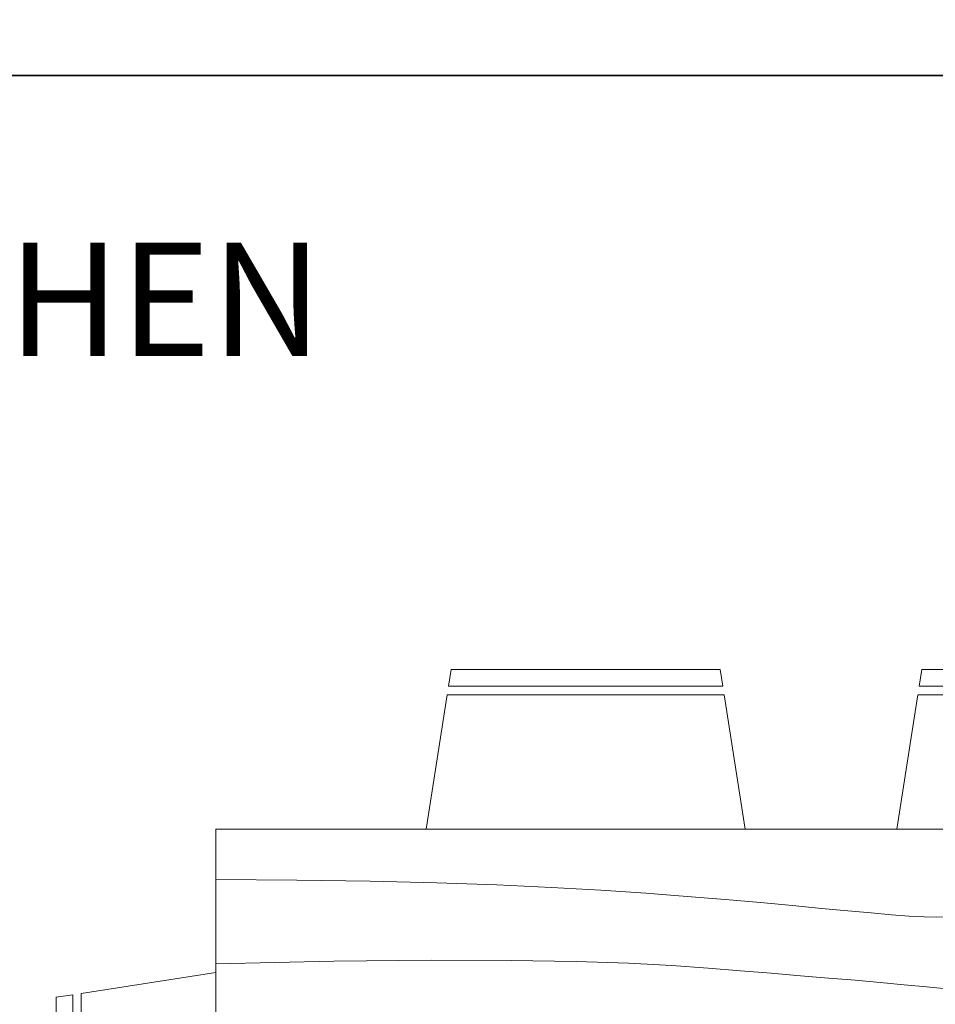
# Model space of a CAD drawing. Units: inches. Extents: x 4159 to 4826, y 299 to 1026.
# Tile 24 of 37: x 4305 to 4354, y 611 to 663. Entities that reach past the tile are written whole.
import ezdxf

# ---------------------------------------------------------------- set-up
doc = ezdxf.new("R2010")
doc.units = ezdxf.units.IN
for name, color, linetype, lineweight in [('A-ANNO-DIMS', 2, 'Continuous', 18), ('A-AREA-IDEN', 7, 'Continuous', 18), ('A-FURN', 8, 'Continuous', 18), ('A-WALL', 7, 'Continuous', 35)]:
    doc.layers.add(name, color=color, linetype=linetype, lineweight=lineweight)
doc.styles.get("Standard").update_dxf_attribs({"font": 'arial.ttf'})
doc.dimstyles.get("Standard").update_dxf_attribs({"dimtxt": 0.18, "dimasz": 0.18, "dimexe": 0.18, "dimexo": 0.0625, "dimgap": 0.09, "dimtad": 0, "dimtih": 1, "dimtoh": 1, "dimdec": 4, "dimzin": 0, "dimdsep": 46, "dimtxsty": 'Standard', "dimcen": 0.09, "dimadec": 0, "dimazin": 0, "dimtfac": 1, "dimtdec": 4, "dimtofl": 0, "dimtmove": 0, "dimatfit": 3, "dimfxl": 1, "dimtolj": 1, "dimtzin": 0, "dimarcsym": 0})

# ---------------------------------------------------------------- blocks, each defined once
blk = doc.blocks.new('Dining Set - 36 x 72 in.')
for p, q in [((-22, 27.5), (-22.1562, 26.50042)), ((-22, 27.5), (-6, 27.5)), ((-5.8437, 26.49966), (-6, 27.5)), ((6, 27.5), (5.8438, 26.50042)), ((6, 27.5), (22, 27.5)), ((22.1563, 26.49966), (22, 27.5)), ((-5.8416, 26.5), (-22.1534, 26.5)), ((22.1584, 26.5), (5.8466, 26.5)), ((-22.2343, 26.00059), (-23.4847, 17.99762)), ((-22.2304, 26), (-5.7608, 26)), ((-4.5152, 17.99762), (-5.7655, 25.99926)), ((5.7657, 26.00059), (4.5153, 17.99762)), ((5.7696, 26), (22.2392, 26)), ((23.4848, 17.99762), (22.2345, 25.99926)), ((36, 18), (-36, 18)), ((-36, 18), (-36, -18)), ((36, -18), (36, 18)), ((-44.0006, 8.23428), (-35.9976, 9.48474)), ((44.0006, 8.23428), (35.9976, 9.48474)), ((-44, 8.23041), (-44, -8.23915)), ((44, 8.23041), (44, -8.23915)), ((-45.5, 8), (-44.5004, 8.15617)), ((-45.5, 8), (-45.5, -8)), ((-44.5, -8.15843), (-44.5, 8.15338)), ((44.5, -8.15843), (44.5, 8.15338)), ((45.5, 8), (44.5005, 8.15617)), ((45.5, 8), (45.5, -8)), ((-44.4997, -8.15631), (-45.5, -8)), ((44.4997, -8.15631), (45.5, -8)), ((-35.9976, -9.48476), (-43.9993, -8.2345)), ((35.9976, -9.48476), (43.9993, -8.2345)), ((-36, -18), (36, -18)), ((-22.2343, -26.0006), (-23.4847, -17.99762)), ((-4.5152, -17.99762), (-5.7655, -25.99928)), ((5.7657, -26.0006), (4.5153, -17.99762)), ((23.4848, -17.99762), (22.2345, -25.99928)), ((-22.2304, -26), (-5.7608, -26)), ((5.7696, -26), (22.2392, -26)), ((-22, -27.5), (-22.1562, -26.50044)), ((-5.8416, -26.5), (-22.1534, -26.5)), ((-5.8437, -26.49967), (-6, -27.5)), ((6, -27.5), (5.8438, -26.50044)), ((22.1584, -26.5), (5.8466, -26.5)), ((22.1563, -26.49967), (22, -27.5)), ((-22, -27.5), (-6, -27.5)), ((6, -27.5), (22, -27.5))]:
    blk.add_line(p, q)
for points in [[(-36, 15), (-31.1772, 14.97754), (-26.8079, 14.91406), (-22.8538, 14.81543), (-19.276, 14.6875), (-16.0362, 14.53613), (-13.0957, 14.36718), (-10.4159, 14.18652), (-7.9583, 14), (-5.6904, 13.81315), (-3.6035, 13.63021), (-1.6954, 13.45508), (0.0365, 13.29166), (1.5945, 13.14388), (2.9811, 13.01562), (4.1988, 12.9108), (5.25, 12.83333), (6.1393, 12.78613), (6.8802, 12.76823), (7.4883, 12.77767), (7.9792, 12.8125), (8.3685, 12.87077), (8.6719, 12.95052), (8.9049, 13.0498), (9.0833, 13.16666), (9.2205, 13.29899), (9.3216, 13.44401), (9.3895, 13.59879), (9.4271, 13.76041), (9.4373, 13.92594), (9.4232, 14.09245), (9.3875, 14.257), (9.3333, 14.41666), (9.2638, 14.56917), (9.1836, 14.71484), (9.0975, 14.85465), (9.0104, 14.98958), (8.9272, 15.1206), (8.8529, 15.2487), (8.7922, 15.37483), (8.75, 15.5), (8.7305, 15.62467), (8.7344, 15.74739), (8.7617, 15.86621), (8.8125, 15.97916), (8.8867, 16.08431), (8.9844, 16.17968), (9.1055, 16.26334), (9.25, 16.33333), (9.4189, 16.38802), (9.6172, 16.42708), (9.8506, 16.45052), (10.125, 16.45833), (10.4463, 16.45052), (10.8203, 16.42708), (11.2529, 16.38802), (11.75, 16.33333), (12.3184, 16.26318), (12.9694, 16.17838), (13.7151, 16.07991), (14.5677, 15.96875), (15.5395, 15.84586), (16.6426, 15.71224), (17.8893, 15.56884), (19.2917, 15.41666), (20.859, 15.25667), (22.5879, 15.08984), (24.4721, 14.91715), (26.5052, 14.73958), (28.6809, 14.5581), (30.9929, 14.3737), (33.4347, 14.18733), (36, 14)], [(-36, 10), (-28.9766, 10.14274), (-23.1725, 10.20442), (-18.4241, 10.19775), (-14.5677, 10.13541), (-11.4399, 10.03011), (-8.877, 9.89453), (-6.7154, 9.74137), (-4.7917, 9.58333), (-2.9698, 9.43082), (-1.2246, 9.28515), (0.4415, 9.14534), (2.026, 9.01041), (3.5266, 8.87939), (4.9408, 8.7513), (6.266, 8.62516), (7.5, 8.5), (8.6411, 8.37549), (9.6914, 8.2539), (10.6538, 8.13818), (11.5312, 8.03125), (12.3267, 7.93603), (13.043, 7.85547), (13.6831, 7.79248), (14.25, 7.75), (14.7471, 7.7303), (15.1797, 7.73307), (15.5537, 7.75732), (15.875, 7.80208), (16.1494, 7.86637), (16.3828, 7.94922), (16.5811, 8.04964), (16.75, 8.16666), (16.8944, 8.29915), (17.0143, 8.44531), (17.1089, 8.60319), (17.1771, 8.77083), (17.218, 8.94629), (17.2305, 9.1276), (17.2137, 9.31282), (17.1667, 9.5), (17.0895, 9.6875), (16.987, 9.875), (16.8649, 10.0625), (16.7292, 10.25), (16.5856, 10.4375), (16.4401, 10.625), (16.2985, 10.8125), (16.1667, 11), (16.05, 11.18733), (15.9518, 11.3737), (15.8752, 11.5581), (15.8229, 11.73958), (15.798, 11.91715), (15.8034, 12.08984), (15.842, 12.25667), (15.9167, 12.41666), (16.0295, 12.56836), (16.1784, 12.70833), (16.3605, 12.83268), (16.5729, 12.9375), (16.8127, 13.01888), (17.0768, 13.07291), (17.3625, 13.0957), (17.6667, 13.08333), (17.9894, 13.03312), (18.3418, 12.94726), (18.7382, 12.82918), (19.1927, 12.68229), (19.7195, 12.51001), (20.3327, 12.31575), (21.0465, 12.10294), (21.875, 11.875), (22.8357, 11.63354), (23.959, 11.37304), (25.2786, 11.08618), (26.8282, 10.76562), (28.6414, 10.40405), (30.752, 9.99414), (33.1936, 9.52856), (36, 9)], [(-36, 5.5), (-30.7157, 5.3348), (-26.069, 5.20963), (-21.9946, 5.11767), (-18.4271, 5.05208), (-15.3009, 5.00602), (-12.5508, 4.97265), (-10.1112, 4.94515), (-7.9167, 4.91666), (-5.909, 4.88167), (-4.0586, 4.83984), (-2.3429, 4.79215), (-0.7396, 4.73958), (0.7739, 4.6831), (2.22, 4.6237), (3.6213, 4.56233), (5, 4.5), (6.373, 4.43782), (7.7344, 4.3776), (9.0723, 4.32129), (10.375, 4.27083), (11.6309, 4.22819), (12.8281, 4.19531), (13.9551, 4.17415), (15, 4.16666), (15.954, 4.17448), (16.819, 4.19791), (17.6001, 4.23698), (18.3021, 4.29166), (18.9299, 4.36198), (19.4883, 4.44791), (19.9823, 4.54948), (20.4167, 4.66666), (20.7969, 4.79899), (21.1302, 4.94401), (21.4245, 5.09879), (21.6875, 5.26041), (21.9271, 5.42594), (22.1511, 5.59245), (22.3672, 5.757), (22.5834, 5.91666), (22.8065, 6.06868), (23.0404, 6.21093), (23.2879, 6.34147), (23.5521, 6.45833), (23.8358, 6.55957), (24.142, 6.64323), (24.4735, 6.70735), (24.8334, 6.75), (25.2235, 6.76969), (25.642, 6.76692), (26.0858, 6.74267), (26.5521, 6.69791), (27.0379, 6.63362), (27.5404, 6.55078), (28.0565, 6.45036), (28.5834, 6.33333), (29.1242, 6.19987), (29.7071, 6.04687), (30.3661, 5.87044), (31.1354, 5.66666), (32.0493, 5.43164), (33.142, 5.16146), (34.4475, 4.85221), (36, 4.5)], [(-36, -1), (-30.7915, -0.6591), (-26.0195, -0.38216), (-21.6519, -0.16284), (-17.6563, 0.00521), (-14.0005, 0.12833), (-10.6523, 0.21289), (-7.5796, 0.26522), (-4.75, 0.29166), (-2.134, 0.29793), (0.2878, 0.28711), (2.5317, 0.26163), (4.6146, 0.22396), (6.5529, 0.17651), (8.3633, 0.12174), (10.0623, 0.06209), (11.6667, 0), (13.1899, -0.06201), (14.6341, -0.1211), (15.9982, -0.17432), (17.2813, -0.21875), (18.4823, -0.25147), (19.6003, -0.26953), (20.6343, -0.27002), (21.5834, -0.25), (22.4481, -0.20768), (23.2357, -0.14584), (23.9549, -0.06836), (24.6146, 0.02083), (25.2235, 0.11784), (25.7904, 0.21875), (26.3241, 0.31966), (26.8334, 0.41666), (27.3265, 0.50618), (27.8099, 0.58593), (28.2894, 0.65397), (28.7709, 0.70833), (29.2601, 0.74707), (29.763, 0.76823), (30.2855, 0.76985), (30.8334, 0.75), (31.4088, 0.70784), (31.9994, 0.64713), (32.589, 0.57275), (33.1615, 0.48958), (33.7008, 0.4025), (34.1908, 0.3164), (34.6153, 0.23616), (34.9584, 0.16666), (35.2099, 0.11165), (35.3848, 0.07031), (35.504, 0.04069), (35.5886, 0.02083), (35.6594, 0.00879), (35.7377, 0.0026), (35.8442, 0.00032), (36, 0)], [(-36, -6.5), (-27.1843, -6.31267), (-20.084, -6.1263), (-14.469, -5.9419), (-10.1094, -5.76042), (-6.7752, -5.58285), (-4.2363, -5.41016), (-2.2629, -5.24333), (-0.625, -5.08334), (0.8708, -4.93099), (2.2715, -4.78646), (3.5872, -4.64974), (4.8281, -4.52084), (6.0046, -4.39974), (7.127, -4.28646), (8.2053, -4.18099), (9.25, -4.08334), (10.2705, -3.99382), (11.2734, -3.91407), (12.2647, -3.84603), (13.25, -3.79167), (14.2354, -3.75293), (15.2266, -3.73177), (16.2295, -3.73015), (17.25, -3.75), (18.2912, -3.79248), (19.3451, -3.85547), (20.4009, -3.93604), (21.4479, -4.03125), (22.4754, -4.13819), (23.4727, -4.25391), (24.4289, -4.37549), (25.3334, -4.5), (26.1785, -4.62492), (26.9694, -4.74935), (27.7145, -4.87281), (28.4219, -4.99479), (29.1, -5.11483), (29.7572, -5.23242), (30.4016, -5.34709), (31.0417, -5.45834), (31.6837, -5.56437), (32.3262, -5.65821), (32.9658, -5.73153), (33.599, -5.77604), (34.2224, -5.78345), (34.8327, -5.74545), (35.4264, -5.65373), (36, -5.5)], [(-36, -10), (-26.4022, -9.81299), (-18.4675, -9.62891), (-11.9839, -9.45069), (-6.7396, -9.28125), (-2.5226, -9.12354), (0.8789, -8.98047), (3.6769, -8.85498), (6.0833, -8.75), (8.2767, -8.66765), (10.3021, -8.60677), (12.1712, -8.56543), (13.8958, -8.54167), (15.4876, -8.53353), (16.9583, -8.53907), (18.3197, -8.55632), (19.5834, -8.58334), (20.7616, -8.61841), (21.8685, -8.66081), (22.9188, -8.71004), (23.9271, -8.76563), (24.9081, -8.82707), (25.8763, -8.89388), (26.8465, -8.96558), (27.8334, -9.04167), (28.8474, -9.12118), (29.8828, -9.20117), (30.93, -9.27824), (31.9792, -9.34896), (33.0205, -9.40991), (34.0443, -9.45768), (35.0407, -9.48885), (36, -9.5)], [(-36, -14.5), (-30.0881, -14.33513), (-25.0332, -14.21224), (-20.7312, -14.12647), (-17.0781, -14.07292), (-13.97, -14.04671), (-11.3027, -14.04297), (-8.9724, -14.05681), (-6.875, -14.08334), (-4.9224, -14.11833), (-3.0905, -14.16016), (-1.3709, -14.20785), (0.2448, -14.26042), (1.7647, -14.3169), (3.1973, -14.3763), (4.5507, -14.43767), (5.8333, -14.5), (7.0554, -14.5621), (8.235, -14.62175), (9.3922, -14.67652), (10.5469, -14.72396), (11.7192, -14.76164), (12.929, -14.78711), (14.1965, -14.79794), (15.5417, -14.79167), (16.9933, -14.76424), (18.6152, -14.70508), (20.4804, -14.60197), (22.6615, -14.44271), (25.2312, -14.21509), (28.2624, -13.9069), (31.8277, -13.50594), (36, -13)]]:
    blk.add_lwpolyline(points)
blk = doc.blocks.new('*D44')
at = {"layer": 'A-ANNO-DIMS', "color": 0, "lineweight": -2, "transparency": 16777216}
for p, q in [((4287.263, 963.093), (4158.88, 963.093)), ((4159.06, 962.913), (4159.06, 647.826)), ((4159.06, 332.375), (4159.06, 647.462)), ((4447.248, 332.195), (4158.88, 332.195))]:
    blk.add_line(p, q, dxfattribs=at)
at = {"layer": 'A-ANNO-DIMS', "color": 0, "transparency": 16777216}
for points in [[(4159.03, 962.913), (4159.09, 962.913), (4159.06, 963.093)], [(4159.03, 332.375), (4159.09, 332.375), (4159.06, 332.195)]]:
    blk.add_solid(points, dxfattribs=at)
at = {"layer": 'Defpoints', "color": 0, "transparency": 16777216}
for p in [(4287.326, 963.093), (4159.06, 332.195), (4447.31, 332.195)]:
    blk.add_point(p, dxfattribs=at)
at = {"layer": 'A-ANNO-DIMS', "color": 0, "transparency": 16777216, "insert": (4159.06, 647.644), "char_height": 0.18, "attachment_point": 5}
blk.add_mtext('\\A1;630.9', dxfattribs=at)

msp = doc.modelspace()

# ---------------------------------------------------------------- linework, layer by layer
at = {"layer": 'A-WALL'}
msp.add_line((4447.31, 660.254), (4201.31, 660.254), dxfattribs=at)

# ---------------------------------------------------------------- block references
at = {"layer": 'A-FURN', "xscale": 0.8913588978043845, "yscale": 0.8913588978043845, "zscale": 0.8913588978043845}
msp.add_blockref('Dining Set - 36 x 72 in.', (4347.717, 604.246), dxfattribs=at)

# ---------------------------------------------------------------- texts
at = {"layer": 'A-AREA-IDEN'}
msp.add_text('OPEN KITCHEN', height=6, dxfattribs=at).set_placement((4262.954, 645.382))

# ---------------------------------------------------------------- dimensions: what is measured, and where the dimension line sits
at = {"layer": 'A-ANNO-DIMS'}
dim = msp.add_linear_dim(base=(4159.06, 332.195), p1=(4287.326, 963.093), p2=(4447.31, 332.195), angle=90, dimstyle='Standard', override={"dimdec": 1, "dimlfac": 1, "dimrnd": 0, "dimzin": 0, "dimdsep": 46, "dimlunit": 2}, dxfattribs=at)
dim.commit()
dim.dimension.update_dxf_attribs({"geometry": '*D44', "text_midpoint": (4159.06, 647.644)})

doc.saveas('drawing.dxf')
